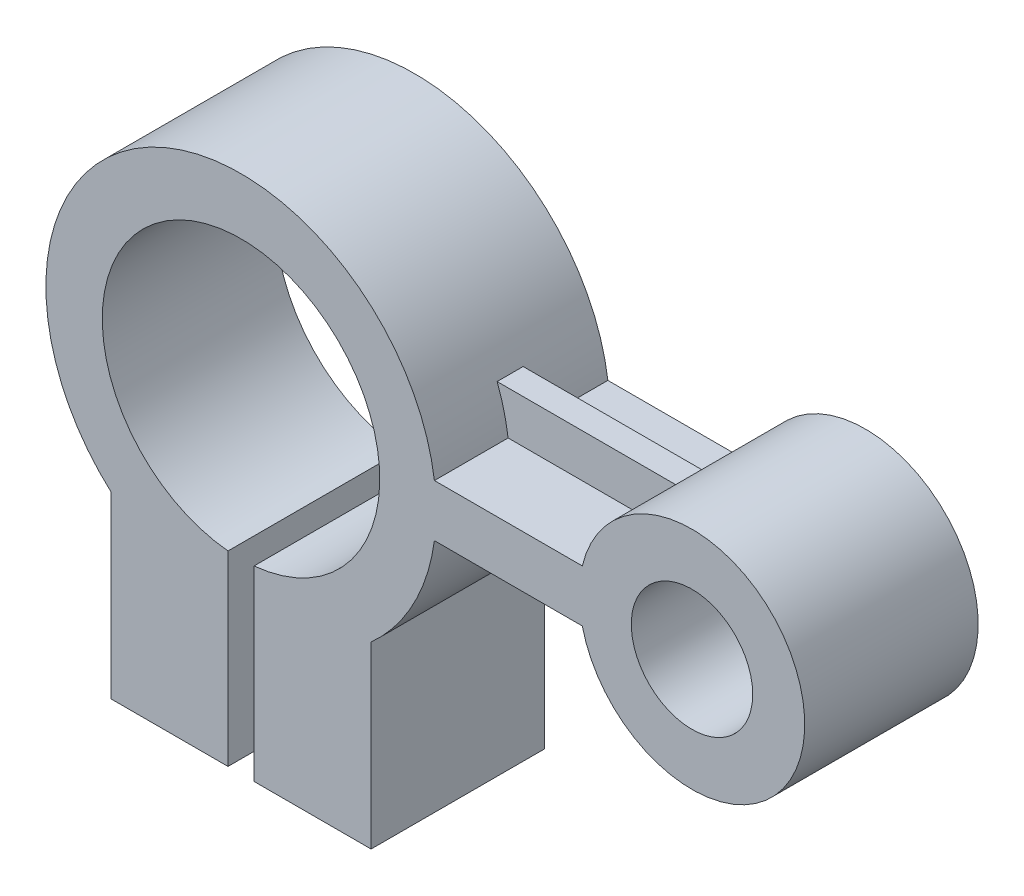
ISO-10303-21;
HEADER;
FILE_DESCRIPTION(('STEP AP214'),'2;1');
FILE_NAME('part.step','',(''),(''),'','','');
FILE_SCHEMA(('AUTOMOTIVE_DESIGN { 1 0 10303 214 1 1 1 1 }'));
ENDSEC;
DATA;
#1=APPLICATION_CONTEXT('core data for automotive mechanical design processes');
#2=APPLICATION_PROTOCOL_DEFINITION('international standard','automotive_design',2000,#1);
#3=PRODUCT_CONTEXT('',#1,'mechanical');
#4=PRODUCT('Part','Part','',(#3));
#5=PRODUCT_RELATED_PRODUCT_CATEGORY('part','',(#4));
#6=PRODUCT_DEFINITION_FORMATION('','',#4);
#7=PRODUCT_DEFINITION_CONTEXT('part definition',#1,'design');
#8=PRODUCT_DEFINITION('design','',#6,#7);
#9=PRODUCT_DEFINITION_SHAPE('','',#8);
#10=(LENGTH_UNIT() NAMED_UNIT(*) SI_UNIT(.MILLI.,.METRE.));
#11=(NAMED_UNIT(*) PLANE_ANGLE_UNIT() SI_UNIT($,.RADIAN.));
#12=(NAMED_UNIT(*) SI_UNIT($,.STERADIAN.) SOLID_ANGLE_UNIT());
#13=UNCERTAINTY_MEASURE_WITH_UNIT(LENGTH_MEASURE(1.E-05),#10,'distance_accuracy_value','');
#14=(GEOMETRIC_REPRESENTATION_CONTEXT(3) GLOBAL_UNCERTAINTY_ASSIGNED_CONTEXT((#13)) GLOBAL_UNIT_ASSIGNED_CONTEXT((#10,
#11,#12)) REPRESENTATION_CONTEXT('',''));
#15=CARTESIAN_POINT('',(0.,0.,0.));
#16=DIRECTION('',(0.,0.,1.));
#17=DIRECTION('',(1.,0.,0.));
#18=AXIS2_PLACEMENT_3D('',#15,#16,#17);
#19=CARTESIAN_POINT('',(104.,0.,40.));
#20=DIRECTION('',(0.,0.,-1.));
#21=DIRECTION('',(-1.,0.,0.));
#22=AXIS2_PLACEMENT_3D('',#19,#20,#21);
#23=CYLINDRICAL_SURFACE('',#22,26.);
#24=CARTESIAN_POINT('',(104.,0.,23.));
#25=DIRECTION('',(0.,0.,-1.));
#26=DIRECTION('',(-1.,0.,0.));
#27=AXIS2_PLACEMENT_3D('',#24,#25,#26);
#28=CIRCLE('',#27,26.);
#29=CARTESIAN_POINT('',(83.5060984680808,-16.,23.));
#30=VERTEX_POINT('',#29);
#31=CARTESIAN_POINT('',(78.701778718653,-6.,23.));
#32=VERTEX_POINT('',#31);
#33=EDGE_CURVE('E63',#30,#32,#28,.T.);
#34=ORIENTED_EDGE('',*,*,#33,.F.);
#35=DIRECTION('',(0.,0.,-1.));
#36=VECTOR('',#35,1.);
#37=CARTESIAN_POINT('',(83.5060984680808,-16.,40.));
#38=LINE('',#37,#36);
#39=CARTESIAN_POINT('',(83.5060984680808,-16.,20.));
#40=VERTEX_POINT('',#39);
#41=EDGE_CURVE('E58',#30,#40,#38,.T.);
#42=ORIENTED_EDGE('',*,*,#41,.T.);
#43=CARTESIAN_POINT('',(104.,0.,20.));
#44=DIRECTION('',(0.,0.,1.));
#45=DIRECTION('',(1.,0.,0.));
#46=AXIS2_PLACEMENT_3D('',#43,#44,#45);
#47=CIRCLE('',#46,26.);
#48=CARTESIAN_POINT('',(78.701778718653,-6.,20.));
#49=VERTEX_POINT('',#48);
#50=EDGE_CURVE('E195',#49,#40,#47,.T.);
#51=ORIENTED_EDGE('',*,*,#50,.F.);
#52=DIRECTION('',(0.,0.,-1.));
#53=VECTOR('',#52,1.);
#54=CARTESIAN_POINT('',(78.701778718653,-6.,40.));
#55=LINE('',#54,#53);
#56=CARTESIAN_POINT('',(78.701778718653,-6.,0.));
#57=VERTEX_POINT('',#56);
#58=EDGE_CURVE('E179',#49,#57,#55,.T.);
#59=ORIENTED_EDGE('',*,*,#58,.T.);
#60=CARTESIAN_POINT('',(104.,0.,0.));
#61=DIRECTION('',(0.,0.,1.));
#62=DIRECTION('',(1.,0.,0.));
#63=AXIS2_PLACEMENT_3D('',#60,#61,#62);
#64=CIRCLE('',#63,26.);
#65=CARTESIAN_POINT('',(78.701778718653,6.,0.));
#66=VERTEX_POINT('',#65);
#67=EDGE_CURVE('E231',#57,#66,#64,.T.);
#68=ORIENTED_EDGE('',*,*,#67,.T.);
#69=DIRECTION('',(0.,0.,-1.));
#70=VECTOR('',#69,1.);
#71=CARTESIAN_POINT('',(78.701778718653,6.,40.));
#72=LINE('',#71,#70);
#73=CARTESIAN_POINT('',(78.701778718653,6.,17.));
#74=VERTEX_POINT('',#73);
#75=EDGE_CURVE('E217',#74,#66,#72,.T.);
#76=ORIENTED_EDGE('',*,*,#75,.F.);
#77=CARTESIAN_POINT('',(104.,0.,17.));
#78=DIRECTION('',(0.,0.,1.));
#79=DIRECTION('',(1.,0.,0.));
#80=AXIS2_PLACEMENT_3D('',#77,#78,#79);
#81=CIRCLE('',#80,26.);
#82=CARTESIAN_POINT('',(83.5060984680808,16.,17.));
#83=VERTEX_POINT('',#82);
#84=EDGE_CURVE('E309',#83,#74,#81,.T.);
#85=ORIENTED_EDGE('',*,*,#84,.F.);
#86=DIRECTION('',(0.,0.,-1.));
#87=VECTOR('',#86,1.);
#88=CARTESIAN_POINT('',(83.5060984680808,16.,40.));
#89=LINE('',#88,#87);
#90=CARTESIAN_POINT('',(83.5060984680808,16.,23.));
#91=VERTEX_POINT('',#90);
#92=EDGE_CURVE('E312',#91,#83,#89,.T.);
#93=ORIENTED_EDGE('',*,*,#92,.F.);
#94=CARTESIAN_POINT('',(104.,0.,23.));
#95=DIRECTION('',(0.,0.,-1.));
#96=DIRECTION('',(-1.,0.,0.));
#97=AXIS2_PLACEMENT_3D('',#94,#95,#96);
#98=CIRCLE('',#97,26.);
#99=CARTESIAN_POINT('',(78.701778718653,6.,23.));
#100=VERTEX_POINT('',#99);
#101=EDGE_CURVE('E302',#100,#91,#98,.T.);
#102=ORIENTED_EDGE('',*,*,#101,.F.);
#103=CARTESIAN_POINT('',(78.701778718653,6.,40.));
#104=VERTEX_POINT('',#103);
#105=EDGE_CURVE('E214',#104,#100,#72,.T.);
#106=ORIENTED_EDGE('',*,*,#105,.F.);
#107=CARTESIAN_POINT('',(104.,0.,40.));
#108=DIRECTION('',(0.,0.,1.));
#109=DIRECTION('',(1.,0.,0.));
#110=AXIS2_PLACEMENT_3D('',#107,#108,#109);
#111=CIRCLE('',#110,26.);
#112=CARTESIAN_POINT('',(78.701778718653,-6.,40.));
#113=VERTEX_POINT('',#112);
#114=EDGE_CURVE('E228',#113,#104,#111,.T.);
#115=ORIENTED_EDGE('',*,*,#114,.F.);
#116=EDGE_CURVE('E186',#113,#32,#55,.T.);
#117=ORIENTED_EDGE('',*,*,#116,.T.);
#118=EDGE_LOOP('',(#34,#42,#51,#59,#68,#76,#85,#93,#102,#106,#115,#117));
#119=FACE_BOUND('',#118,.T.);
#120=ADVANCED_FACE('F46',(#119),#23,.T.);
#121=CARTESIAN_POINT('',(0.,0.,40.));
#122=DIRECTION('',(0.,0.,-1.));
#123=DIRECTION('',(-1.,0.,0.));
#124=AXIS2_PLACEMENT_3D('',#121,#122,#123);
#125=CYLINDRICAL_SURFACE('',#124,45.);
#126=CARTESIAN_POINT('',(0.,0.,23.));
#127=DIRECTION('',(0.,0.,-1.));
#128=DIRECTION('',(-1.,0.,0.));
#129=AXIS2_PLACEMENT_3D('',#126,#127,#128);
#130=CIRCLE('',#129,45.);
#131=CARTESIAN_POINT('',(44.5982062419555,-6.,23.));
#132=VERTEX_POINT('',#131);
#133=CARTESIAN_POINT('',(42.0594816896262,-16.,23.));
#134=VERTEX_POINT('',#133);
#135=EDGE_CURVE('E197',#132,#134,#130,.T.);
#136=ORIENTED_EDGE('',*,*,#135,.F.);
#137=DIRECTION('',(0.,0.,-1.));
#138=VECTOR('',#137,1.);
#139=CARTESIAN_POINT('',(44.5982062419555,-6.,40.));
#140=LINE('',#139,#138);
#141=CARTESIAN_POINT('',(44.5982062419555,-6.,40.));
#142=VERTEX_POINT('',#141);
#143=EDGE_CURVE('E224',#142,#132,#140,.T.);
#144=ORIENTED_EDGE('',*,*,#143,.F.);
#145=CARTESIAN_POINT('',(0.,0.,40.));
#146=DIRECTION('',(0.,0.,1.));
#147=DIRECTION('',(1.,0.,0.));
#148=AXIS2_PLACEMENT_3D('',#145,#146,#147);
#149=CIRCLE('',#148,45.);
#150=CARTESIAN_POINT('',(30.,-33.5410196624969,40.));
#151=VERTEX_POINT('',#150);
#152=EDGE_CURVE('E239',#151,#142,#149,.T.);
#153=ORIENTED_EDGE('',*,*,#152,.F.);
#154=DIRECTION('',(0.,0.,1.));
#155=VECTOR('',#154,1.);
#156=CARTESIAN_POINT('',(30.,-33.5410196624969,0.));
#157=LINE('',#156,#155);
#158=CARTESIAN_POINT('',(30.,-33.5410196624969,0.));
#159=VERTEX_POINT('',#158);
#160=EDGE_CURVE('E283',#159,#151,#157,.T.);
#161=ORIENTED_EDGE('',*,*,#160,.F.);
#162=CARTESIAN_POINT('',(0.,0.,0.));
#163=DIRECTION('',(0.,0.,1.));
#164=DIRECTION('',(1.,0.,0.));
#165=AXIS2_PLACEMENT_3D('',#162,#163,#164);
#166=CIRCLE('',#165,45.);
#167=CARTESIAN_POINT('',(44.5982062419555,-6.,0.));
#168=VERTEX_POINT('',#167);
#169=EDGE_CURVE('E230',#159,#168,#166,.T.);
#170=ORIENTED_EDGE('',*,*,#169,.T.);
#171=CARTESIAN_POINT('',(44.5982062419555,-6.,20.));
#172=VERTEX_POINT('',#171);
#173=EDGE_CURVE('E225',#172,#168,#140,.T.);
#174=ORIENTED_EDGE('',*,*,#173,.F.);
#175=CARTESIAN_POINT('',(0.,0.,20.));
#176=DIRECTION('',(0.,0.,1.));
#177=DIRECTION('',(1.,0.,0.));
#178=AXIS2_PLACEMENT_3D('',#175,#176,#177);
#179=CIRCLE('',#178,45.);
#180=CARTESIAN_POINT('',(42.0594816896262,-16.,20.));
#181=VERTEX_POINT('',#180);
#182=EDGE_CURVE('E200',#181,#172,#179,.T.);
#183=ORIENTED_EDGE('',*,*,#182,.F.);
#184=DIRECTION('',(0.,0.,-1.));
#185=VECTOR('',#184,1.);
#186=CARTESIAN_POINT('',(42.0594816896262,-16.,40.));
#187=LINE('',#186,#185);
#188=EDGE_CURVE('E12',#181,#134,#187,.F.);
#189=ORIENTED_EDGE('',*,*,#188,.T.);
#190=EDGE_LOOP('',(#136,#144,#153,#161,#170,#174,#183,#189));
#191=FACE_BOUND('',#190,.T.);
#192=ADVANCED_FACE('F343',(#191),#125,.T.);
#193=CARTESIAN_POINT('',(52.,-6.,40.));
#194=DIRECTION('',(0.,1.,0.));
#195=DIRECTION('',(0.,0.,1.));
#196=AXIS2_PLACEMENT_3D('',#193,#194,#195);
#197=PLANE('',#196);
#198=DIRECTION('',(-1.,0.,0.));
#199=VECTOR('',#198,1.);
#200=CARTESIAN_POINT('',(52.,-6.,23.));
#201=LINE('',#200,#199);
#202=EDGE_CURVE('E52',#32,#132,#201,.T.);
#203=ORIENTED_EDGE('',*,*,#202,.F.);
#204=ORIENTED_EDGE('',*,*,#116,.F.);
#205=DIRECTION('',(1.,0.,0.));
#206=VECTOR('',#205,1.);
#207=CARTESIAN_POINT('',(44.5982062419555,-6.,40.));
#208=LINE('',#207,#206);
#209=EDGE_CURVE('E188',#142,#113,#208,.T.);
#210=ORIENTED_EDGE('',*,*,#209,.F.);
#211=ORIENTED_EDGE('',*,*,#143,.T.);
#212=EDGE_LOOP('',(#203,#204,#210,#211));
#213=FACE_BOUND('',#212,.T.);
#214=ADVANCED_FACE('F346',(#213),#197,.F.);
#215=DIRECTION('',(1.,0.,0.));
#216=VECTOR('',#215,1.);
#217=CARTESIAN_POINT('',(52.,-6.,20.));
#218=LINE('',#217,#216);
#219=EDGE_CURVE('E182',#172,#49,#218,.T.);
#220=ORIENTED_EDGE('',*,*,#219,.F.);
#221=ORIENTED_EDGE('',*,*,#173,.T.);
#222=DIRECTION('',(1.,0.,0.));
#223=VECTOR('',#222,1.);
#224=CARTESIAN_POINT('',(52.,-6.,0.));
#225=LINE('',#224,#223);
#226=EDGE_CURVE('E187',#168,#57,#225,.T.);
#227=ORIENTED_EDGE('',*,*,#226,.T.);
#228=ORIENTED_EDGE('',*,*,#58,.F.);
#229=EDGE_LOOP('',(#220,#221,#227,#228));
#230=FACE_BOUND('',#229,.T.);
#231=ADVANCED_FACE('F181',(#230),#197,.F.);
#232=CARTESIAN_POINT('',(52.,6.,40.));
#233=DIRECTION('',(0.,-1.,0.));
#234=DIRECTION('',(0.,0.,-1.));
#235=AXIS2_PLACEMENT_3D('',#232,#233,#234);
#236=PLANE('',#235);
#237=DIRECTION('',(1.,0.,0.));
#238=VECTOR('',#237,1.);
#239=CARTESIAN_POINT('',(88.9472240076308,6.,23.));
#240=LINE('',#239,#238);
#241=CARTESIAN_POINT('',(44.5982062419555,6.,23.));
#242=VERTEX_POINT('',#241);
#243=EDGE_CURVE('E322',#242,#100,#240,.T.);
#244=ORIENTED_EDGE('',*,*,#243,.F.);
#245=DIRECTION('',(0.,0.,-1.));
#246=VECTOR('',#245,1.);
#247=CARTESIAN_POINT('',(44.5982062419555,6.,40.));
#248=LINE('',#247,#246);
#249=CARTESIAN_POINT('',(44.5982062419555,6.,40.));
#250=VERTEX_POINT('',#249);
#251=EDGE_CURVE('E220',#250,#242,#248,.T.);
#252=ORIENTED_EDGE('',*,*,#251,.F.);
#253=DIRECTION('',(-1.,0.,0.));
#254=VECTOR('',#253,1.);
#255=CARTESIAN_POINT('',(52.,6.,40.));
#256=LINE('',#255,#254);
#257=EDGE_CURVE('E241',#104,#250,#256,.T.);
#258=ORIENTED_EDGE('',*,*,#257,.F.);
#259=ORIENTED_EDGE('',*,*,#105,.T.);
#260=EDGE_LOOP('',(#244,#252,#258,#259));
#261=FACE_BOUND('',#260,.T.);
#262=ADVANCED_FACE('F378',(#261),#236,.F.);
#263=DIRECTION('',(-1.,0.,0.));
#264=VECTOR('',#263,1.);
#265=CARTESIAN_POINT('',(32.9126005820921,6.,17.));
#266=LINE('',#265,#264);
#267=CARTESIAN_POINT('',(44.5982062419555,6.,17.));
#268=VERTEX_POINT('',#267);
#269=EDGE_CURVE('E320',#74,#268,#266,.T.);
#270=ORIENTED_EDGE('',*,*,#269,.F.);
#271=ORIENTED_EDGE('',*,*,#75,.T.);
#272=DIRECTION('',(-1.,0.,0.));
#273=VECTOR('',#272,1.);
#274=CARTESIAN_POINT('',(52.,6.,0.));
#275=LINE('',#274,#273);
#276=CARTESIAN_POINT('',(44.5982062419555,6.,0.));
#277=VERTEX_POINT('',#276);
#278=EDGE_CURVE('E229',#66,#277,#275,.T.);
#279=ORIENTED_EDGE('',*,*,#278,.T.);
#280=EDGE_CURVE('E218',#268,#277,#248,.T.);
#281=ORIENTED_EDGE('',*,*,#280,.F.);
#282=EDGE_LOOP('',(#270,#271,#279,#281));
#283=FACE_BOUND('',#282,.T.);
#284=ADVANCED_FACE('F406',(#283),#236,.F.);
#285=CARTESIAN_POINT('',(0.,0.,23.));
#286=DIRECTION('',(0.,0.,-1.));
#287=DIRECTION('',(-1.,0.,0.));
#288=AXIS2_PLACEMENT_3D('',#285,#286,#287);
#289=CIRCLE('',#288,45.);
#290=CARTESIAN_POINT('',(42.0594816896262,16.,23.));
#291=VERTEX_POINT('',#290);
#292=EDGE_CURVE('E204',#291,#242,#289,.T.);
#293=ORIENTED_EDGE('',*,*,#292,.F.);
#294=DIRECTION('',(0.,0.,-1.));
#295=VECTOR('',#294,1.);
#296=CARTESIAN_POINT('',(42.0594816896262,16.,40.));
#297=LINE('',#296,#295);
#298=CARTESIAN_POINT('',(42.0594816896262,16.,17.));
#299=VERTEX_POINT('',#298);
#300=EDGE_CURVE('E208',#299,#291,#297,.F.);
#301=ORIENTED_EDGE('',*,*,#300,.F.);
#302=CARTESIAN_POINT('',(0.,0.,17.));
#303=DIRECTION('',(0.,0.,1.));
#304=DIRECTION('',(1.,0.,0.));
#305=AXIS2_PLACEMENT_3D('',#302,#303,#304);
#306=CIRCLE('',#305,45.);
#307=EDGE_CURVE('E202',#268,#299,#306,.T.);
#308=ORIENTED_EDGE('',*,*,#307,.F.);
#309=ORIENTED_EDGE('',*,*,#280,.T.);
#310=CARTESIAN_POINT('',(-30.,-33.5410196624969,0.));
#311=VERTEX_POINT('',#310);
#312=EDGE_CURVE('E227',#277,#311,#166,.T.);
#313=ORIENTED_EDGE('',*,*,#312,.T.);
#314=DIRECTION('',(0.,0.,1.));
#315=VECTOR('',#314,1.);
#316=CARTESIAN_POINT('',(-30.,-33.5410196624969,0.));
#317=LINE('',#316,#315);
#318=CARTESIAN_POINT('',(-30.,-33.5410196624969,40.));
#319=VERTEX_POINT('',#318);
#320=EDGE_CURVE('E272',#311,#319,#317,.T.);
#321=ORIENTED_EDGE('',*,*,#320,.T.);
#322=EDGE_CURVE('E240',#250,#319,#149,.T.);
#323=ORIENTED_EDGE('',*,*,#322,.F.);
#324=ORIENTED_EDGE('',*,*,#251,.T.);
#325=EDGE_LOOP('',(#293,#301,#308,#309,#313,#321,#323,#324));
#326=FACE_BOUND('',#325,.T.);
#327=ADVANCED_FACE('F385',(#326),#125,.T.);
#328=CARTESIAN_POINT('',(104.,0.,40.));
#329=DIRECTION('',(0.,0.,1.));
#330=DIRECTION('',(1.,0.,0.));
#331=AXIS2_PLACEMENT_3D('',#328,#329,#330);
#332=PLANE('',#331);
#333=DIRECTION('',(0.,1.,0.));
#334=VECTOR('',#333,1.);
#335=CARTESIAN_POINT('',(3.,0.,40.));
#336=LINE('',#335,#334);
#337=CARTESIAN_POINT('',(3.,-74.8998886412873,40.));
#338=VERTEX_POINT('',#337);
#339=CARTESIAN_POINT('',(3.,-31.859064644148,40.));
#340=VERTEX_POINT('',#339);
#341=EDGE_CURVE('E253',#338,#340,#336,.T.);
#342=ORIENTED_EDGE('',*,*,#341,.F.);
#343=DIRECTION('',(1.,0.,0.));
#344=VECTOR('',#343,1.);
#345=CARTESIAN_POINT('',(3.,-74.8998886412873,40.));
#346=LINE('',#345,#344);
#347=CARTESIAN_POINT('',(30.,-74.8998886412873,40.));
#348=VERTEX_POINT('',#347);
#349=EDGE_CURVE('E301',#338,#348,#346,.T.);
#350=ORIENTED_EDGE('',*,*,#349,.T.);
#351=DIRECTION('',(0.,1.,0.));
#352=VECTOR('',#351,1.);
#353=CARTESIAN_POINT('',(30.,-74.8998886412873,40.));
#354=LINE('',#353,#352);
#355=EDGE_CURVE('E300',#348,#151,#354,.T.);
#356=ORIENTED_EDGE('',*,*,#355,.T.);
#357=ORIENTED_EDGE('',*,*,#152,.T.);
#358=ORIENTED_EDGE('',*,*,#209,.T.);
#359=ORIENTED_EDGE('',*,*,#114,.T.);
#360=ORIENTED_EDGE('',*,*,#257,.T.);
#361=ORIENTED_EDGE('',*,*,#322,.T.);
#362=DIRECTION('',(0.,-1.,0.));
#363=VECTOR('',#362,1.);
#364=CARTESIAN_POINT('',(-30.,-74.8998886412873,40.));
#365=LINE('',#364,#363);
#366=CARTESIAN_POINT('',(-30.,-74.8998886412873,40.));
#367=VERTEX_POINT('',#366);
#368=EDGE_CURVE('E285',#319,#367,#365,.T.);
#369=ORIENTED_EDGE('',*,*,#368,.T.);
#370=DIRECTION('',(1.,0.,0.));
#371=VECTOR('',#370,1.);
#372=CARTESIAN_POINT('',(-3.,-74.8998886412873,40.));
#373=LINE('',#372,#371);
#374=CARTESIAN_POINT('',(-3.,-74.8998886412873,40.));
#375=VERTEX_POINT('',#374);
#376=EDGE_CURVE('E279',#367,#375,#373,.T.);
#377=ORIENTED_EDGE('',*,*,#376,.T.);
#378=DIRECTION('',(0.,-1.,0.));
#379=VECTOR('',#378,1.);
#380=CARTESIAN_POINT('',(-3.,0.,40.));
#381=LINE('',#380,#379);
#382=CARTESIAN_POINT('',(-3.,-31.859064644148,40.));
#383=VERTEX_POINT('',#382);
#384=EDGE_CURVE('E256',#383,#375,#381,.T.);
#385=ORIENTED_EDGE('',*,*,#384,.F.);
#386=CARTESIAN_POINT('',(0.,0.,40.));
#387=DIRECTION('',(0.,0.,1.));
#388=DIRECTION('',(1.,0.,0.));
#389=AXIS2_PLACEMENT_3D('',#386,#387,#388);
#390=CIRCLE('',#389,32.);
#391=EDGE_CURVE('E262',#340,#383,#390,.T.);
#392=ORIENTED_EDGE('',*,*,#391,.F.);
#393=EDGE_LOOP('',(#342,#350,#356,#357,#358,#359,#360,#361,#369,#377,#385,#392));
#394=FACE_BOUND('',#393,.T.);
#395=CARTESIAN_POINT('',(104.,0.,40.));
#396=DIRECTION('',(0.,0.,1.));
#397=DIRECTION('',(1.,0.,0.));
#398=AXIS2_PLACEMENT_3D('',#395,#396,#397);
#399=CIRCLE('',#398,14.);
#400=CARTESIAN_POINT('',(118.,0.,40.));
#401=VERTEX_POINT('',#400);
#402=EDGE_CURVE('E244',#401,#401,#399,.T.);
#403=ORIENTED_EDGE('',*,*,#402,.F.);
#404=EDGE_LOOP('',(#403));
#405=FACE_BOUND('',#404,.T.);
#406=ADVANCED_FACE('F355',(#394,#405),#332,.T.);
#407=CARTESIAN_POINT('',(104.,0.,0.));
#408=DIRECTION('',(0.,0.,1.));
#409=DIRECTION('',(1.,0.,0.));
#410=AXIS2_PLACEMENT_3D('',#407,#408,#409);
#411=PLANE('',#410);
#412=CARTESIAN_POINT('',(104.,0.,0.));
#413=DIRECTION('',(0.,0.,1.));
#414=DIRECTION('',(1.,0.,0.));
#415=AXIS2_PLACEMENT_3D('',#412,#413,#414);
#416=CIRCLE('',#415,14.);
#417=CARTESIAN_POINT('',(118.,0.,0.));
#418=VERTEX_POINT('',#417);
#419=EDGE_CURVE('E232',#418,#418,#416,.T.);
#420=ORIENTED_EDGE('',*,*,#419,.T.);
#421=EDGE_LOOP('',(#420));
#422=FACE_BOUND('',#421,.T.);
#423=ORIENTED_EDGE('',*,*,#169,.F.);
#424=DIRECTION('',(0.,1.,0.));
#425=VECTOR('',#424,1.);
#426=CARTESIAN_POINT('',(30.,-74.8998886412873,0.));
#427=LINE('',#426,#425);
#428=CARTESIAN_POINT('',(30.,-74.8998886412873,0.));
#429=VERTEX_POINT('',#428);
#430=EDGE_CURVE('E295',#429,#159,#427,.T.);
#431=ORIENTED_EDGE('',*,*,#430,.F.);
#432=DIRECTION('',(1.,0.,0.));
#433=VECTOR('',#432,1.);
#434=CARTESIAN_POINT('',(3.,-74.8998886412873,0.));
#435=LINE('',#434,#433);
#436=CARTESIAN_POINT('',(3.,-74.8998886412873,0.));
#437=VERTEX_POINT('',#436);
#438=EDGE_CURVE('E297',#437,#429,#435,.T.);
#439=ORIENTED_EDGE('',*,*,#438,.F.);
#440=DIRECTION('',(0.,1.,0.));
#441=VECTOR('',#440,1.);
#442=CARTESIAN_POINT('',(3.,0.,0.));
#443=LINE('',#442,#441);
#444=CARTESIAN_POINT('',(3.,-31.859064644148,0.));
#445=VERTEX_POINT('',#444);
#446=EDGE_CURVE('E254',#437,#445,#443,.T.);
#447=ORIENTED_EDGE('',*,*,#446,.T.);
#448=CARTESIAN_POINT('',(0.,0.,0.));
#449=DIRECTION('',(0.,0.,1.));
#450=DIRECTION('',(1.,0.,0.));
#451=AXIS2_PLACEMENT_3D('',#448,#449,#450);
#452=CIRCLE('',#451,32.);
#453=CARTESIAN_POINT('',(-3.,-31.859064644148,0.));
#454=VERTEX_POINT('',#453);
#455=EDGE_CURVE('E259',#445,#454,#452,.T.);
#456=ORIENTED_EDGE('',*,*,#455,.T.);
#457=DIRECTION('',(0.,-1.,0.));
#458=VECTOR('',#457,1.);
#459=CARTESIAN_POINT('',(-3.,0.,0.));
#460=LINE('',#459,#458);
#461=CARTESIAN_POINT('',(-3.,-74.8998886412873,0.));
#462=VERTEX_POINT('',#461);
#463=EDGE_CURVE('E266',#454,#462,#460,.T.);
#464=ORIENTED_EDGE('',*,*,#463,.T.);
#465=DIRECTION('',(1.,0.,0.));
#466=VECTOR('',#465,1.);
#467=CARTESIAN_POINT('',(-3.,-74.8998886412873,0.));
#468=LINE('',#467,#466);
#469=CARTESIAN_POINT('',(-30.,-74.8998886412873,0.));
#470=VERTEX_POINT('',#469);
#471=EDGE_CURVE('E274',#470,#462,#468,.T.);
#472=ORIENTED_EDGE('',*,*,#471,.F.);
#473=DIRECTION('',(0.,-1.,0.));
#474=VECTOR('',#473,1.);
#475=CARTESIAN_POINT('',(-30.,-74.8998886412873,0.));
#476=LINE('',#475,#474);
#477=EDGE_CURVE('E282',#311,#470,#476,.T.);
#478=ORIENTED_EDGE('',*,*,#477,.F.);
#479=ORIENTED_EDGE('',*,*,#312,.F.);
#480=ORIENTED_EDGE('',*,*,#278,.F.);
#481=ORIENTED_EDGE('',*,*,#67,.F.);
#482=ORIENTED_EDGE('',*,*,#226,.F.);
#483=EDGE_LOOP('',(#423,#431,#439,#447,#456,#464,#472,#478,#479,#480,#481,#482));
#484=FACE_BOUND('',#483,.T.);
#485=ADVANCED_FACE('F361',(#422,#484),#411,.F.);
#486=CARTESIAN_POINT('',(104.,0.,0.));
#487=DIRECTION('',(0.,0.,1.));
#488=DIRECTION('',(1.,0.,0.));
#489=AXIS2_PLACEMENT_3D('',#486,#487,#488);
#490=CYLINDRICAL_SURFACE('',#489,14.);
#491=ORIENTED_EDGE('',*,*,#419,.F.);
#492=EDGE_LOOP('',(#491));
#493=FACE_BOUND('',#492,.T.);
#494=ORIENTED_EDGE('',*,*,#402,.T.);
#495=EDGE_LOOP('',(#494));
#496=FACE_BOUND('',#495,.T.);
#497=ADVANCED_FACE('F427',(#493,#496),#490,.F.);
#498=CARTESIAN_POINT('',(0.,0.,0.));
#499=DIRECTION('',(0.,0.,1.));
#500=DIRECTION('',(1.,0.,0.));
#501=AXIS2_PLACEMENT_3D('',#498,#499,#500);
#502=CYLINDRICAL_SURFACE('',#501,32.);
#503=ORIENTED_EDGE('',*,*,#391,.T.);
#504=DIRECTION('',(0.,0.,1.));
#505=VECTOR('',#504,1.);
#506=CARTESIAN_POINT('',(-3.,-31.859064644148,0.));
#507=LINE('',#506,#505);
#508=EDGE_CURVE('E252',#454,#383,#507,.T.);
#509=ORIENTED_EDGE('',*,*,#508,.F.);
#510=ORIENTED_EDGE('',*,*,#455,.F.);
#511=DIRECTION('',(0.,0.,1.));
#512=VECTOR('',#511,1.);
#513=CARTESIAN_POINT('',(3.,-31.859064644148,0.));
#514=LINE('',#513,#512);
#515=EDGE_CURVE('E247',#445,#340,#514,.T.);
#516=ORIENTED_EDGE('',*,*,#515,.T.);
#517=EDGE_LOOP('',(#503,#509,#510,#516));
#518=FACE_BOUND('',#517,.T.);
#519=ADVANCED_FACE('F397',(#518),#502,.F.);
#520=CARTESIAN_POINT('',(3.,0.,0.));
#521=DIRECTION('',(1.,0.,0.));
#522=DIRECTION('',(0.,0.,-1.));
#523=AXIS2_PLACEMENT_3D('',#520,#521,#522);
#524=PLANE('',#523);
#525=ORIENTED_EDGE('',*,*,#341,.T.);
#526=ORIENTED_EDGE('',*,*,#515,.F.);
#527=ORIENTED_EDGE('',*,*,#446,.F.);
#528=DIRECTION('',(0.,0.,1.));
#529=VECTOR('',#528,1.);
#530=CARTESIAN_POINT('',(3.,-74.8998886412873,0.));
#531=LINE('',#530,#529);
#532=EDGE_CURVE('E287',#437,#338,#531,.T.);
#533=ORIENTED_EDGE('',*,*,#532,.T.);
#534=EDGE_LOOP('',(#525,#526,#527,#533));
#535=FACE_BOUND('',#534,.T.);
#536=ADVANCED_FACE('F405',(#535),#524,.F.);
#537=CARTESIAN_POINT('',(-3.,0.,0.));
#538=DIRECTION('',(-1.,0.,0.));
#539=DIRECTION('',(0.,0.,1.));
#540=AXIS2_PLACEMENT_3D('',#537,#538,#539);
#541=PLANE('',#540);
#542=ORIENTED_EDGE('',*,*,#384,.T.);
#543=DIRECTION('',(0.,0.,1.));
#544=VECTOR('',#543,1.);
#545=CARTESIAN_POINT('',(-3.,-74.8998886412873,0.));
#546=LINE('',#545,#544);
#547=EDGE_CURVE('E261',#462,#375,#546,.T.);
#548=ORIENTED_EDGE('',*,*,#547,.F.);
#549=ORIENTED_EDGE('',*,*,#463,.F.);
#550=ORIENTED_EDGE('',*,*,#508,.T.);
#551=EDGE_LOOP('',(#542,#548,#549,#550));
#552=FACE_BOUND('',#551,.T.);
#553=ADVANCED_FACE('F399',(#552),#541,.F.);
#554=CARTESIAN_POINT('',(-3.,-74.8998886412873,0.));
#555=DIRECTION('',(0.,-1.,0.));
#556=DIRECTION('',(0.,0.,-1.));
#557=AXIS2_PLACEMENT_3D('',#554,#555,#556);
#558=PLANE('',#557);
#559=ORIENTED_EDGE('',*,*,#376,.F.);
#560=DIRECTION('',(0.,0.,1.));
#561=VECTOR('',#560,1.);
#562=CARTESIAN_POINT('',(-30.,-74.8998886412873,0.));
#563=LINE('',#562,#561);
#564=EDGE_CURVE('E271',#470,#367,#563,.T.);
#565=ORIENTED_EDGE('',*,*,#564,.F.);
#566=ORIENTED_EDGE('',*,*,#471,.T.);
#567=ORIENTED_EDGE('',*,*,#547,.T.);
#568=EDGE_LOOP('',(#559,#565,#566,#567));
#569=FACE_BOUND('',#568,.T.);
#570=ADVANCED_FACE('F392',(#569),#558,.T.);
#571=CARTESIAN_POINT('',(-30.,-74.8998886412873,0.));
#572=DIRECTION('',(-1.,0.,0.));
#573=DIRECTION('',(0.,0.,1.));
#574=AXIS2_PLACEMENT_3D('',#571,#572,#573);
#575=PLANE('',#574);
#576=ORIENTED_EDGE('',*,*,#368,.F.);
#577=ORIENTED_EDGE('',*,*,#320,.F.);
#578=ORIENTED_EDGE('',*,*,#477,.T.);
#579=ORIENTED_EDGE('',*,*,#564,.T.);
#580=EDGE_LOOP('',(#576,#577,#578,#579));
#581=FACE_BOUND('',#580,.T.);
#582=ADVANCED_FACE('F387',(#581),#575,.T.);
#583=CARTESIAN_POINT('',(30.,-74.8998886412873,0.));
#584=DIRECTION('',(1.,0.,0.));
#585=DIRECTION('',(0.,0.,-1.));
#586=AXIS2_PLACEMENT_3D('',#583,#584,#585);
#587=PLANE('',#586);
#588=ORIENTED_EDGE('',*,*,#355,.F.);
#589=DIRECTION('',(0.,0.,1.));
#590=VECTOR('',#589,1.);
#591=CARTESIAN_POINT('',(30.,-74.8998886412873,0.));
#592=LINE('',#591,#590);
#593=EDGE_CURVE('E291',#429,#348,#592,.T.);
#594=ORIENTED_EDGE('',*,*,#593,.F.);
#595=ORIENTED_EDGE('',*,*,#430,.T.);
#596=ORIENTED_EDGE('',*,*,#160,.T.);
#597=EDGE_LOOP('',(#588,#594,#595,#596));
#598=FACE_BOUND('',#597,.T.);
#599=ADVANCED_FACE('F407',(#598),#587,.T.);
#600=CARTESIAN_POINT('',(3.,-74.8998886412873,0.));
#601=DIRECTION('',(0.,-1.,0.));
#602=DIRECTION('',(0.,0.,-1.));
#603=AXIS2_PLACEMENT_3D('',#600,#601,#602);
#604=PLANE('',#603);
#605=ORIENTED_EDGE('',*,*,#349,.F.);
#606=ORIENTED_EDGE('',*,*,#532,.F.);
#607=ORIENTED_EDGE('',*,*,#438,.T.);
#608=ORIENTED_EDGE('',*,*,#593,.T.);
#609=EDGE_LOOP('',(#605,#606,#607,#608));
#610=FACE_BOUND('',#609,.T.);
#611=ADVANCED_FACE('F410',(#610),#604,.T.);
#612=CARTESIAN_POINT('',(0.,16.,0.));
#613=DIRECTION('',(0.,-1.,0.));
#614=DIRECTION('',(0.,0.,-1.));
#615=AXIS2_PLACEMENT_3D('',#612,#613,#614);
#616=PLANE('',#615);
#617=DIRECTION('',(1.,0.,0.));
#618=VECTOR('',#617,1.);
#619=CARTESIAN_POINT('',(88.9472240076308,16.,23.));
#620=LINE('',#619,#618);
#621=EDGE_CURVE('E318',#291,#91,#620,.T.);
#622=ORIENTED_EDGE('',*,*,#621,.T.);
#623=ORIENTED_EDGE('',*,*,#92,.T.);
#624=DIRECTION('',(-1.,0.,0.));
#625=VECTOR('',#624,1.);
#626=CARTESIAN_POINT('',(32.9126005820921,16.,17.));
#627=LINE('',#626,#625);
#628=EDGE_CURVE('E317',#83,#299,#627,.T.);
#629=ORIENTED_EDGE('',*,*,#628,.T.);
#630=ORIENTED_EDGE('',*,*,#300,.T.);
#631=EDGE_LOOP('',(#622,#623,#629,#630));
#632=FACE_BOUND('',#631,.T.);
#633=ADVANCED_FACE('F373',(#632),#616,.F.);
#634=CARTESIAN_POINT('',(88.9472240076308,16.,23.));
#635=DIRECTION('',(0.,0.,-1.));
#636=DIRECTION('',(-1.,0.,0.));
#637=AXIS2_PLACEMENT_3D('',#634,#635,#636);
#638=PLANE('',#637);
#639=ORIENTED_EDGE('',*,*,#243,.T.);
#640=ORIENTED_EDGE('',*,*,#101,.T.);
#641=ORIENTED_EDGE('',*,*,#621,.F.);
#642=ORIENTED_EDGE('',*,*,#292,.T.);
#643=EDGE_LOOP('',(#639,#640,#641,#642));
#644=FACE_BOUND('',#643,.T.);
#645=ADVANCED_FACE('F376',(#644),#638,.F.);
#646=CARTESIAN_POINT('',(32.9126005820921,16.,17.));
#647=DIRECTION('',(0.,0.,1.));
#648=DIRECTION('',(1.,0.,0.));
#649=AXIS2_PLACEMENT_3D('',#646,#647,#648);
#650=PLANE('',#649);
#651=ORIENTED_EDGE('',*,*,#628,.F.);
#652=ORIENTED_EDGE('',*,*,#84,.T.);
#653=ORIENTED_EDGE('',*,*,#269,.T.);
#654=ORIENTED_EDGE('',*,*,#307,.T.);
#655=EDGE_LOOP('',(#651,#652,#653,#654));
#656=FACE_BOUND('',#655,.T.);
#657=ADVANCED_FACE('F371',(#656),#650,.F.);
#658=CARTESIAN_POINT('',(0.,-16.,0.));
#659=DIRECTION('',(0.,-1.,0.));
#660=DIRECTION('',(0.,0.,-1.));
#661=AXIS2_PLACEMENT_3D('',#658,#659,#660);
#662=PLANE('',#661);
#663=ORIENTED_EDGE('',*,*,#41,.F.);
#664=DIRECTION('',(-1.,0.,0.));
#665=VECTOR('',#664,1.);
#666=CARTESIAN_POINT('',(86.3404810812223,-16.,23.));
#667=LINE('',#666,#665);
#668=EDGE_CURVE('E332',#30,#134,#667,.T.);
#669=ORIENTED_EDGE('',*,*,#668,.T.);
#670=ORIENTED_EDGE('',*,*,#188,.F.);
#671=DIRECTION('',(1.,0.,0.));
#672=VECTOR('',#671,1.);
#673=CARTESIAN_POINT('',(37.4933327740208,-16.,20.));
#674=LINE('',#673,#672);
#675=EDGE_CURVE('E335',#181,#40,#674,.T.);
#676=ORIENTED_EDGE('',*,*,#675,.T.);
#677=EDGE_LOOP('',(#663,#669,#670,#676));
#678=FACE_BOUND('',#677,.T.);
#679=ADVANCED_FACE('F338',(#678),#662,.T.);
#680=CARTESIAN_POINT('',(44.5982062419555,-16.,23.));
#681=DIRECTION('',(0.,0.,-1.));
#682=DIRECTION('',(-1.,0.,0.));
#683=AXIS2_PLACEMENT_3D('',#680,#681,#682);
#684=PLANE('',#683);
#685=ORIENTED_EDGE('',*,*,#668,.F.);
#686=ORIENTED_EDGE('',*,*,#33,.T.);
#687=ORIENTED_EDGE('',*,*,#202,.T.);
#688=ORIENTED_EDGE('',*,*,#135,.T.);
#689=EDGE_LOOP('',(#685,#686,#687,#688));
#690=FACE_BOUND('',#689,.T.);
#691=ADVANCED_FACE('F345',(#690),#684,.F.);
#692=CARTESIAN_POINT('',(37.4933327740208,-16.,20.));
#693=DIRECTION('',(0.,0.,1.));
#694=DIRECTION('',(1.,0.,0.));
#695=AXIS2_PLACEMENT_3D('',#692,#693,#694);
#696=PLANE('',#695);
#697=ORIENTED_EDGE('',*,*,#219,.T.);
#698=ORIENTED_EDGE('',*,*,#50,.T.);
#699=ORIENTED_EDGE('',*,*,#675,.F.);
#700=ORIENTED_EDGE('',*,*,#182,.T.);
#701=EDGE_LOOP('',(#697,#698,#699,#700));
#702=FACE_BOUND('',#701,.T.);
#703=ADVANCED_FACE('F198',(#702),#696,.F.);
#704=CLOSED_SHELL('',(#120,#192,#214,#231,#262,#284,#327,#406,#485,#497,#519,#536,#553,#570,
#582,#599,#611,#633,#645,#657,#679,#691,#703));
#705=MANIFOLD_SOLID_BREP('B2',#704);
#706=ADVANCED_BREP_SHAPE_REPRESENTATION('',(#18,#705),#14);
#707=SHAPE_DEFINITION_REPRESENTATION(#9,#706);
ENDSEC;
END-ISO-10303-21;
